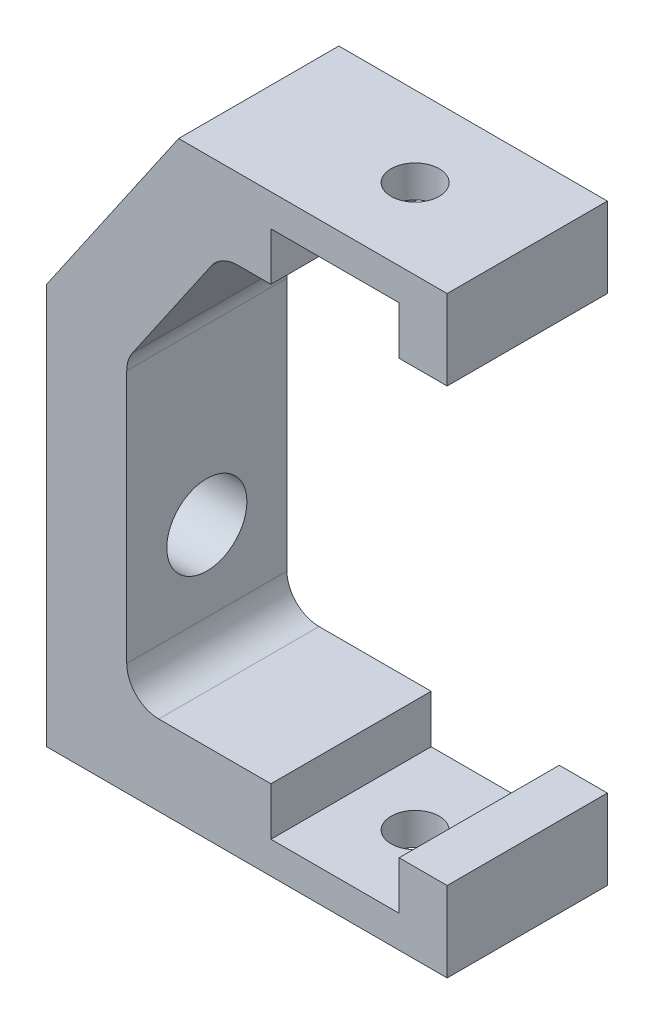
ISO-10303-21;
HEADER;
FILE_DESCRIPTION(('STEP AP214'),'2;1');
FILE_NAME('part.step','',(''),(''),'','','');
FILE_SCHEMA(('AUTOMOTIVE_DESIGN { 1 0 10303 214 1 1 1 1 }'));
ENDSEC;
DATA;
#1=APPLICATION_CONTEXT('core data for automotive mechanical design processes');
#2=APPLICATION_PROTOCOL_DEFINITION('international standard','automotive_design',2000,#1);
#3=PRODUCT_CONTEXT('',#1,'mechanical');
#4=PRODUCT('Part','Part','',(#3));
#5=PRODUCT_RELATED_PRODUCT_CATEGORY('part','',(#4));
#6=PRODUCT_DEFINITION_FORMATION('','',#4);
#7=PRODUCT_DEFINITION_CONTEXT('part definition',#1,'design');
#8=PRODUCT_DEFINITION('design','',#6,#7);
#9=PRODUCT_DEFINITION_SHAPE('','',#8);
#10=(LENGTH_UNIT() NAMED_UNIT(*) SI_UNIT(.MILLI.,.METRE.));
#11=(NAMED_UNIT(*) PLANE_ANGLE_UNIT() SI_UNIT($,.RADIAN.));
#12=(NAMED_UNIT(*) SI_UNIT($,.STERADIAN.) SOLID_ANGLE_UNIT());
#13=UNCERTAINTY_MEASURE_WITH_UNIT(LENGTH_MEASURE(1.E-05),#10,'distance_accuracy_value','');
#14=(GEOMETRIC_REPRESENTATION_CONTEXT(3) GLOBAL_UNCERTAINTY_ASSIGNED_CONTEXT((#13)) GLOBAL_UNIT_ASSIGNED_CONTEXT((#10,
#11,#12)) REPRESENTATION_CONTEXT('',''));
#15=CARTESIAN_POINT('',(0.,0.,0.));
#16=DIRECTION('',(0.,0.,1.));
#17=DIRECTION('',(1.,0.,0.));
#18=AXIS2_PLACEMENT_3D('',#15,#16,#17);
#19=CARTESIAN_POINT('',(25.,0.,5.));
#20=DIRECTION('',(0.,1.,0.));
#21=DIRECTION('',(0.,0.,1.));
#22=AXIS2_PLACEMENT_3D('',#19,#20,#21);
#23=PLANE('',#22);
#24=CARTESIAN_POINT('',(18.,0.,0.));
#25=DIRECTION('',(0.,1.,0.));
#26=DIRECTION('',(0.,0.,1.));
#27=AXIS2_PLACEMENT_3D('',#24,#25,#26);
#28=CIRCLE('',#27,1.5);
#29=CARTESIAN_POINT('',(18.,0.,1.5));
#30=VERTEX_POINT('',#29);
#31=EDGE_CURVE('E388',#30,#30,#28,.T.);
#32=ORIENTED_EDGE('',*,*,#31,.T.);
#33=EDGE_LOOP('',(#32));
#34=FACE_BOUND('',#33,.T.);
#35=DIRECTION('',(1.,0.,0.));
#36=VECTOR('',#35,1.);
#37=CARTESIAN_POINT('',(25.,0.,-5.));
#38=LINE('',#37,#36);
#39=CARTESIAN_POINT('',(0.,0.,-5.));
#40=VERTEX_POINT('',#39);
#41=CARTESIAN_POINT('',(25.,0.,-5.));
#42=VERTEX_POINT('',#41);
#43=EDGE_CURVE('E212',#40,#42,#38,.T.);
#44=ORIENTED_EDGE('',*,*,#43,.T.);
#45=DIRECTION('',(0.,0.,-1.));
#46=VECTOR('',#45,1.);
#47=CARTESIAN_POINT('',(25.,0.,5.));
#48=LINE('',#47,#46);
#49=CARTESIAN_POINT('',(25.,0.,5.));
#50=VERTEX_POINT('',#49);
#51=EDGE_CURVE('E11',#50,#42,#48,.T.);
#52=ORIENTED_EDGE('',*,*,#51,.F.);
#53=DIRECTION('',(1.,0.,0.));
#54=VECTOR('',#53,1.);
#55=CARTESIAN_POINT('',(25.,0.,5.));
#56=LINE('',#55,#54);
#57=CARTESIAN_POINT('',(0.,0.,5.));
#58=VERTEX_POINT('',#57);
#59=EDGE_CURVE('E255',#58,#50,#56,.T.);
#60=ORIENTED_EDGE('',*,*,#59,.F.);
#61=DIRECTION('',(0.,0.,-1.));
#62=VECTOR('',#61,1.);
#63=CARTESIAN_POINT('',(0.,0.,5.));
#64=LINE('',#63,#62);
#65=EDGE_CURVE('E209',#58,#40,#64,.T.);
#66=ORIENTED_EDGE('',*,*,#65,.T.);
#67=EDGE_LOOP('',(#44,#52,#60,#66));
#68=FACE_BOUND('',#67,.T.);
#69=ADVANCED_FACE('F39',(#34,#68),#23,.F.);
#70=CARTESIAN_POINT('',(25.,5.,5.));
#71=DIRECTION('',(-1.,0.,0.));
#72=DIRECTION('',(0.,0.,1.));
#73=AXIS2_PLACEMENT_3D('',#70,#71,#72);
#74=PLANE('',#73);
#75=DIRECTION('',(0.,1.,0.));
#76=VECTOR('',#75,1.);
#77=CARTESIAN_POINT('',(25.,5.,-5.));
#78=LINE('',#77,#76);
#79=CARTESIAN_POINT('',(25.,5.,-5.));
#80=VERTEX_POINT('',#79);
#81=EDGE_CURVE('E220',#42,#80,#78,.T.);
#82=ORIENTED_EDGE('',*,*,#81,.T.);
#83=DIRECTION('',(0.,0.,-1.));
#84=VECTOR('',#83,1.);
#85=CARTESIAN_POINT('',(25.,5.,5.));
#86=LINE('',#85,#84);
#87=CARTESIAN_POINT('',(25.,5.,5.));
#88=VERTEX_POINT('',#87);
#89=EDGE_CURVE('E48',#88,#80,#86,.T.);
#90=ORIENTED_EDGE('',*,*,#89,.F.);
#91=DIRECTION('',(0.,1.,0.));
#92=VECTOR('',#91,1.);
#93=CARTESIAN_POINT('',(25.,5.,5.));
#94=LINE('',#93,#92);
#95=EDGE_CURVE('E137',#50,#88,#94,.T.);
#96=ORIENTED_EDGE('',*,*,#95,.F.);
#97=ORIENTED_EDGE('',*,*,#51,.T.);
#98=EDGE_LOOP('',(#82,#90,#96,#97));
#99=FACE_BOUND('',#98,.T.);
#100=ADVANCED_FACE('F385',(#99),#74,.F.);
#101=CARTESIAN_POINT('',(25.,5.,5.));
#102=DIRECTION('',(0.,-1.,0.));
#103=DIRECTION('',(1.,0.,0.));
#104=AXIS2_PLACEMENT_3D('',#101,#102,#103);
#105=PLANE('',#104);
#106=DIRECTION('',(-1.,0.,0.));
#107=VECTOR('',#106,1.);
#108=CARTESIAN_POINT('',(25.,5.,-5.));
#109=LINE('',#108,#107);
#110=CARTESIAN_POINT('',(22.,5.,-5.));
#111=VERTEX_POINT('',#110);
#112=EDGE_CURVE('E218',#80,#111,#109,.T.);
#113=ORIENTED_EDGE('',*,*,#112,.T.);
#114=DIRECTION('',(0.,0.,-1.));
#115=VECTOR('',#114,1.);
#116=CARTESIAN_POINT('',(22.,5.,5.));
#117=LINE('',#116,#115);
#118=CARTESIAN_POINT('',(22.,5.,5.));
#119=VERTEX_POINT('',#118);
#120=EDGE_CURVE('E300',#119,#111,#117,.T.);
#121=ORIENTED_EDGE('',*,*,#120,.F.);
#122=DIRECTION('',(-1.,0.,0.));
#123=VECTOR('',#122,1.);
#124=CARTESIAN_POINT('',(25.,5.,5.));
#125=LINE('',#124,#123);
#126=EDGE_CURVE('E310',#88,#119,#125,.T.);
#127=ORIENTED_EDGE('',*,*,#126,.F.);
#128=ORIENTED_EDGE('',*,*,#89,.T.);
#129=EDGE_LOOP('',(#113,#121,#127,#128));
#130=FACE_BOUND('',#129,.T.);
#131=ADVANCED_FACE('F307',(#130),#105,.F.);
#132=CARTESIAN_POINT('',(22.,2.,5.));
#133=DIRECTION('',(1.,0.,0.));
#134=DIRECTION('',(0.,0.,-1.));
#135=AXIS2_PLACEMENT_3D('',#132,#133,#134);
#136=PLANE('',#135);
#137=DIRECTION('',(0.,-1.,0.));
#138=VECTOR('',#137,1.);
#139=CARTESIAN_POINT('',(22.,2.,-5.));
#140=LINE('',#139,#138);
#141=CARTESIAN_POINT('',(22.,2.,-5.));
#142=VERTEX_POINT('',#141);
#143=EDGE_CURVE('E222',#111,#142,#140,.T.);
#144=ORIENTED_EDGE('',*,*,#143,.T.);
#145=DIRECTION('',(0.,0.,-1.));
#146=VECTOR('',#145,1.);
#147=CARTESIAN_POINT('',(22.,2.,5.));
#148=LINE('',#147,#146);
#149=CARTESIAN_POINT('',(22.,2.,5.));
#150=VERTEX_POINT('',#149);
#151=EDGE_CURVE('E297',#150,#142,#148,.T.);
#152=ORIENTED_EDGE('',*,*,#151,.F.);
#153=DIRECTION('',(0.,-1.,0.));
#154=VECTOR('',#153,1.);
#155=CARTESIAN_POINT('',(22.,2.,5.));
#156=LINE('',#155,#154);
#157=EDGE_CURVE('E330',#119,#150,#156,.T.);
#158=ORIENTED_EDGE('',*,*,#157,.F.);
#159=ORIENTED_EDGE('',*,*,#120,.T.);
#160=EDGE_LOOP('',(#144,#152,#158,#159));
#161=FACE_BOUND('',#160,.T.);
#162=ADVANCED_FACE('F318',(#161),#136,.F.);
#163=CARTESIAN_POINT('',(14.,2.,5.));
#164=DIRECTION('',(0.,-1.,0.));
#165=DIRECTION('',(0.,0.,-1.));
#166=AXIS2_PLACEMENT_3D('',#163,#164,#165);
#167=PLANE('',#166);
#168=CARTESIAN_POINT('',(18.,2.,0.));
#169=DIRECTION('',(0.,-1.,0.));
#170=DIRECTION('',(0.,0.,-1.));
#171=AXIS2_PLACEMENT_3D('',#168,#169,#170);
#172=CIRCLE('',#171,1.5);
#173=CARTESIAN_POINT('',(18.,2.,-1.5));
#174=VERTEX_POINT('',#173);
#175=EDGE_CURVE('E394',#174,#174,#172,.T.);
#176=ORIENTED_EDGE('',*,*,#175,.T.);
#177=EDGE_LOOP('',(#176));
#178=FACE_BOUND('',#177,.T.);
#179=DIRECTION('',(-1.,0.,0.));
#180=VECTOR('',#179,1.);
#181=CARTESIAN_POINT('',(14.,2.,-5.));
#182=LINE('',#181,#180);
#183=CARTESIAN_POINT('',(14.,2.,-5.));
#184=VERTEX_POINT('',#183);
#185=EDGE_CURVE('E224',#142,#184,#182,.T.);
#186=ORIENTED_EDGE('',*,*,#185,.T.);
#187=DIRECTION('',(0.,0.,-1.));
#188=VECTOR('',#187,1.);
#189=CARTESIAN_POINT('',(14.,2.,5.));
#190=LINE('',#189,#188);
#191=CARTESIAN_POINT('',(14.,2.,5.));
#192=VERTEX_POINT('',#191);
#193=EDGE_CURVE('E294',#192,#184,#190,.T.);
#194=ORIENTED_EDGE('',*,*,#193,.F.);
#195=DIRECTION('',(-1.,0.,0.));
#196=VECTOR('',#195,1.);
#197=CARTESIAN_POINT('',(14.,2.,5.));
#198=LINE('',#197,#196);
#199=EDGE_CURVE('E322',#150,#192,#198,.T.);
#200=ORIENTED_EDGE('',*,*,#199,.F.);
#201=ORIENTED_EDGE('',*,*,#151,.T.);
#202=EDGE_LOOP('',(#186,#194,#200,#201));
#203=FACE_BOUND('',#202,.T.);
#204=ADVANCED_FACE('F325',(#178,#203),#167,.F.);
#205=CARTESIAN_POINT('',(14.,5.,5.));
#206=DIRECTION('',(-1.,0.,0.));
#207=DIRECTION('',(0.,0.,1.));
#208=AXIS2_PLACEMENT_3D('',#205,#206,#207);
#209=PLANE('',#208);
#210=DIRECTION('',(0.,1.,0.));
#211=VECTOR('',#210,1.);
#212=CARTESIAN_POINT('',(14.,5.,-5.));
#213=LINE('',#212,#211);
#214=CARTESIAN_POINT('',(14.,5.,-5.));
#215=VERTEX_POINT('',#214);
#216=EDGE_CURVE('E223',#184,#215,#213,.T.);
#217=ORIENTED_EDGE('',*,*,#216,.T.);
#218=DIRECTION('',(0.,0.,-1.));
#219=VECTOR('',#218,1.);
#220=CARTESIAN_POINT('',(14.,5.,5.));
#221=LINE('',#220,#219);
#222=CARTESIAN_POINT('',(14.,5.,5.));
#223=VERTEX_POINT('',#222);
#224=EDGE_CURVE('E292',#223,#215,#221,.T.);
#225=ORIENTED_EDGE('',*,*,#224,.F.);
#226=DIRECTION('',(0.,1.,0.));
#227=VECTOR('',#226,1.);
#228=CARTESIAN_POINT('',(14.,5.,5.));
#229=LINE('',#228,#227);
#230=EDGE_CURVE('E326',#192,#223,#229,.T.);
#231=ORIENTED_EDGE('',*,*,#230,.F.);
#232=ORIENTED_EDGE('',*,*,#193,.T.);
#233=EDGE_LOOP('',(#217,#225,#231,#232));
#234=FACE_BOUND('',#233,.T.);
#235=ADVANCED_FACE('F458',(#234),#209,.F.);
#236=CARTESIAN_POINT('',(14.,5.,5.));
#237=DIRECTION('',(0.,-1.,0.));
#238=DIRECTION('',(1.,0.,0.));
#239=AXIS2_PLACEMENT_3D('',#236,#237,#238);
#240=PLANE('',#239);
#241=DIRECTION('',(-1.,0.,0.));
#242=VECTOR('',#241,1.);
#243=CARTESIAN_POINT('',(14.,5.,-5.));
#244=LINE('',#243,#242);
#245=CARTESIAN_POINT('',(7.00000000000002,5.,-5.));
#246=VERTEX_POINT('',#245);
#247=EDGE_CURVE('E227',#215,#246,#244,.T.);
#248=ORIENTED_EDGE('',*,*,#247,.T.);
#249=DIRECTION('',(0.,0.,-1.));
#250=VECTOR('',#249,1.);
#251=CARTESIAN_POINT('',(7.00000000000002,5.,5.));
#252=LINE('',#251,#250);
#253=CARTESIAN_POINT('',(7.00000000000002,5.,5.));
#254=VERTEX_POINT('',#253);
#255=EDGE_CURVE('E287',#254,#246,#252,.T.);
#256=ORIENTED_EDGE('',*,*,#255,.F.);
#257=DIRECTION('',(-1.,0.,0.));
#258=VECTOR('',#257,1.);
#259=CARTESIAN_POINT('',(14.,5.,5.));
#260=LINE('',#259,#258);
#261=EDGE_CURVE('E328',#223,#254,#260,.T.);
#262=ORIENTED_EDGE('',*,*,#261,.F.);
#263=ORIENTED_EDGE('',*,*,#224,.T.);
#264=EDGE_LOOP('',(#248,#256,#262,#263));
#265=FACE_BOUND('',#264,.T.);
#266=ADVANCED_FACE('F457',(#265),#240,.F.);
#267=CARTESIAN_POINT('',(7.,7.,5.));
#268=DIRECTION('',(0.,0.,-1.));
#269=DIRECTION('',(-1.,0.,0.));
#270=AXIS2_PLACEMENT_3D('',#267,#268,#269);
#271=CYLINDRICAL_SURFACE('',#270,2.);
#272=CARTESIAN_POINT('',(7.,7.,-5.));
#273=DIRECTION('',(0.,0.,-1.));
#274=DIRECTION('',(-1.,0.,0.));
#275=AXIS2_PLACEMENT_3D('',#272,#273,#274);
#276=CIRCLE('',#275,2.);
#277=CARTESIAN_POINT('',(5.,7.00000000000001,-5.));
#278=VERTEX_POINT('',#277);
#279=EDGE_CURVE('E228',#246,#278,#276,.T.);
#280=ORIENTED_EDGE('',*,*,#279,.T.);
#281=DIRECTION('',(0.,0.,-1.));
#282=VECTOR('',#281,1.);
#283=CARTESIAN_POINT('',(5.,7.00000000000001,5.));
#284=LINE('',#283,#282);
#285=CARTESIAN_POINT('',(5.,7.00000000000001,5.));
#286=VERTEX_POINT('',#285);
#287=EDGE_CURVE('E285',#286,#278,#284,.T.);
#288=ORIENTED_EDGE('',*,*,#287,.F.);
#289=CARTESIAN_POINT('',(7.,7.,5.));
#290=DIRECTION('',(0.,0.,-1.));
#291=DIRECTION('',(-1.,0.,0.));
#292=AXIS2_PLACEMENT_3D('',#289,#290,#291);
#293=CIRCLE('',#292,2.);
#294=EDGE_CURVE('E333',#254,#286,#293,.T.);
#295=ORIENTED_EDGE('',*,*,#294,.F.);
#296=ORIENTED_EDGE('',*,*,#255,.T.);
#297=EDGE_LOOP('',(#280,#288,#295,#296));
#298=FACE_BOUND('',#297,.T.);
#299=ADVANCED_FACE('F454',(#298),#271,.F.);
#300=CARTESIAN_POINT('',(5.,7.00000000000001,5.));
#301=DIRECTION('',(-1.,0.,0.));
#302=DIRECTION('',(0.,0.,1.));
#303=AXIS2_PLACEMENT_3D('',#300,#301,#302);
#304=PLANE('',#303);
#305=CARTESIAN_POINT('',(5.,12.,0.));
#306=DIRECTION('',(1.,0.,0.));
#307=DIRECTION('',(0.,0.,-1.));
#308=AXIS2_PLACEMENT_3D('',#305,#306,#307);
#309=CIRCLE('',#308,2.5);
#310=CARTESIAN_POINT('',(5.,12.,-2.5));
#311=VERTEX_POINT('',#310);
#312=EDGE_CURVE('E392',#311,#311,#309,.T.);
#313=ORIENTED_EDGE('',*,*,#312,.F.);
#314=EDGE_LOOP('',(#313));
#315=FACE_BOUND('',#314,.T.);
#316=DIRECTION('',(0.,1.,0.));
#317=VECTOR('',#316,1.);
#318=CARTESIAN_POINT('',(5.,7.00000000000001,-5.));
#319=LINE('',#318,#317);
#320=CARTESIAN_POINT('',(5.,22.8283399513637,-5.));
#321=VERTEX_POINT('',#320);
#322=EDGE_CURVE('E233',#278,#321,#319,.T.);
#323=ORIENTED_EDGE('',*,*,#322,.T.);
#324=DIRECTION('',(0.,0.,-1.));
#325=VECTOR('',#324,1.);
#326=CARTESIAN_POINT('',(5.,22.8283399513637,5.));
#327=LINE('',#326,#325);
#328=CARTESIAN_POINT('',(5.,22.8283399513637,5.));
#329=VERTEX_POINT('',#328);
#330=EDGE_CURVE('E282',#329,#321,#327,.T.);
#331=ORIENTED_EDGE('',*,*,#330,.F.);
#332=DIRECTION('',(0.,1.,0.));
#333=VECTOR('',#332,1.);
#334=CARTESIAN_POINT('',(5.,7.00000000000001,5.));
#335=LINE('',#334,#333);
#336=EDGE_CURVE('E337',#286,#329,#335,.T.);
#337=ORIENTED_EDGE('',*,*,#336,.F.);
#338=ORIENTED_EDGE('',*,*,#287,.T.);
#339=EDGE_LOOP('',(#323,#331,#337,#338));
#340=FACE_BOUND('',#339,.T.);
#341=ADVANCED_FACE('F448',(#315,#340),#304,.F.);
#342=CARTESIAN_POINT('',(7.,22.8283399513637,5.));
#343=DIRECTION('',(0.,0.,-1.));
#344=DIRECTION('',(-1.,0.,0.));
#345=AXIS2_PLACEMENT_3D('',#342,#343,#344);
#346=CYLINDRICAL_SURFACE('',#345,2.);
#347=CARTESIAN_POINT('',(7.,22.8283399513637,-5.));
#348=DIRECTION('',(0.,0.,-1.));
#349=DIRECTION('',(-1.,0.,0.));
#350=AXIS2_PLACEMENT_3D('',#347,#348,#349);
#351=CIRCLE('',#350,2.);
#352=CARTESIAN_POINT('',(5.35118757467925,23.960337118369,-5.));
#353=VERTEX_POINT('',#352);
#354=EDGE_CURVE('E232',#321,#353,#351,.T.);
#355=ORIENTED_EDGE('',*,*,#354,.T.);
#356=DIRECTION('',(0.,0.,-1.));
#357=VECTOR('',#356,1.);
#358=CARTESIAN_POINT('',(5.35118757467925,23.960337118369,5.));
#359=LINE('',#358,#357);
#360=CARTESIAN_POINT('',(5.35118757467925,23.960337118369,5.));
#361=VERTEX_POINT('',#360);
#362=EDGE_CURVE('E276',#361,#353,#359,.T.);
#363=ORIENTED_EDGE('',*,*,#362,.F.);
#364=CARTESIAN_POINT('',(7.,22.8283399513637,5.));
#365=DIRECTION('',(0.,0.,-1.));
#366=DIRECTION('',(-1.,0.,0.));
#367=AXIS2_PLACEMENT_3D('',#364,#365,#366);
#368=CIRCLE('',#367,2.);
#369=EDGE_CURVE('E338',#329,#361,#368,.T.);
#370=ORIENTED_EDGE('',*,*,#369,.F.);
#371=ORIENTED_EDGE('',*,*,#330,.T.);
#372=EDGE_LOOP('',(#355,#363,#370,#371));
#373=FACE_BOUND('',#372,.T.);
#374=ADVANCED_FACE('F443',(#373),#346,.F.);
#375=CARTESIAN_POINT('',(5.35118757467925,23.960337118369,5.));
#376=DIRECTION('',(-0.824406212660378,0.56599858350262,0.));
#377=DIRECTION('',(-0.56599858350262,-0.824406212660378,0.));
#378=AXIS2_PLACEMENT_3D('',#375,#376,#377);
#379=PLANE('',#378);
#380=DIRECTION('',(0.56599858350262,0.824406212660378,0.));
#381=VECTOR('',#380,1.);
#382=CARTESIAN_POINT('',(5.35118757467925,23.960337118369,-5.));
#383=LINE('',#382,#381);
#384=CARTESIAN_POINT('',(10.2749125133736,31.1319971670052,-5.));
#385=VERTEX_POINT('',#384);
#386=EDGE_CURVE('E231',#353,#385,#383,.T.);
#387=ORIENTED_EDGE('',*,*,#386,.T.);
#388=DIRECTION('',(0.,0.,-1.));
#389=VECTOR('',#388,1.);
#390=CARTESIAN_POINT('',(10.2749125133736,31.1319971670052,5.));
#391=LINE('',#390,#389);
#392=CARTESIAN_POINT('',(10.2749125133736,31.1319971670052,5.));
#393=VERTEX_POINT('',#392);
#394=EDGE_CURVE('E277',#393,#385,#391,.T.);
#395=ORIENTED_EDGE('',*,*,#394,.F.);
#396=DIRECTION('',(0.56599858350262,0.824406212660378,0.));
#397=VECTOR('',#396,1.);
#398=CARTESIAN_POINT('',(5.35118757467925,23.960337118369,5.));
#399=LINE('',#398,#397);
#400=EDGE_CURVE('E343',#361,#393,#399,.T.);
#401=ORIENTED_EDGE('',*,*,#400,.F.);
#402=ORIENTED_EDGE('',*,*,#362,.T.);
#403=EDGE_LOOP('',(#387,#395,#401,#402));
#404=FACE_BOUND('',#403,.T.);
#405=ADVANCED_FACE('F442',(#404),#379,.F.);
#406=CARTESIAN_POINT('',(11.9237249386943,30.,5.));
#407=DIRECTION('',(0.,0.,-1.));
#408=DIRECTION('',(-1.,0.,0.));
#409=AXIS2_PLACEMENT_3D('',#406,#407,#408);
#410=CYLINDRICAL_SURFACE('',#409,2.);
#411=CARTESIAN_POINT('',(11.9237249386943,30.,-5.));
#412=DIRECTION('',(0.,0.,-1.));
#413=DIRECTION('',(1.,0.,0.));
#414=AXIS2_PLACEMENT_3D('',#411,#412,#413);
#415=CIRCLE('',#414,2.);
#416=CARTESIAN_POINT('',(11.9237249386944,32.,-5.));
#417=VERTEX_POINT('',#416);
#418=EDGE_CURVE('E240',#385,#417,#415,.T.);
#419=ORIENTED_EDGE('',*,*,#418,.T.);
#420=DIRECTION('',(0.,0.,-1.));
#421=VECTOR('',#420,1.);
#422=CARTESIAN_POINT('',(11.9237249386944,32.,5.));
#423=LINE('',#422,#421);
#424=CARTESIAN_POINT('',(11.9237249386944,32.,5.));
#425=VERTEX_POINT('',#424);
#426=EDGE_CURVE('E272',#425,#417,#423,.T.);
#427=ORIENTED_EDGE('',*,*,#426,.F.);
#428=CARTESIAN_POINT('',(11.9237249386943,30.,5.));
#429=DIRECTION('',(0.,0.,-1.));
#430=DIRECTION('',(1.,0.,0.));
#431=AXIS2_PLACEMENT_3D('',#428,#429,#430);
#432=CIRCLE('',#431,2.);
#433=EDGE_CURVE('E342',#393,#425,#432,.T.);
#434=ORIENTED_EDGE('',*,*,#433,.F.);
#435=ORIENTED_EDGE('',*,*,#394,.T.);
#436=EDGE_LOOP('',(#419,#427,#434,#435));
#437=FACE_BOUND('',#436,.T.);
#438=ADVANCED_FACE('F440',(#437),#410,.F.);
#439=CARTESIAN_POINT('',(11.9237249386944,32.,5.));
#440=DIRECTION('',(0.,1.,0.));
#441=DIRECTION('',(0.,0.,1.));
#442=AXIS2_PLACEMENT_3D('',#439,#440,#441);
#443=PLANE('',#442);
#444=DIRECTION('',(1.,0.,0.));
#445=VECTOR('',#444,1.);
#446=CARTESIAN_POINT('',(11.9237249386944,32.,-5.));
#447=LINE('',#446,#445);
#448=CARTESIAN_POINT('',(14.,32.,-5.));
#449=VERTEX_POINT('',#448);
#450=EDGE_CURVE('E239',#417,#449,#447,.T.);
#451=ORIENTED_EDGE('',*,*,#450,.T.);
#452=DIRECTION('',(0.,0.,-1.));
#453=VECTOR('',#452,1.);
#454=CARTESIAN_POINT('',(14.,32.,5.));
#455=LINE('',#454,#453);
#456=CARTESIAN_POINT('',(14.,32.,5.));
#457=VERTEX_POINT('',#456);
#458=EDGE_CURVE('E269',#457,#449,#455,.T.);
#459=ORIENTED_EDGE('',*,*,#458,.F.);
#460=DIRECTION('',(1.,0.,0.));
#461=VECTOR('',#460,1.);
#462=CARTESIAN_POINT('',(11.9237249386944,32.,5.));
#463=LINE('',#462,#461);
#464=EDGE_CURVE('E341',#425,#457,#463,.T.);
#465=ORIENTED_EDGE('',*,*,#464,.F.);
#466=ORIENTED_EDGE('',*,*,#426,.T.);
#467=EDGE_LOOP('',(#451,#459,#465,#466));
#468=FACE_BOUND('',#467,.T.);
#469=ADVANCED_FACE('F433',(#468),#443,.F.);
#470=CARTESIAN_POINT('',(14.,35.,5.));
#471=DIRECTION('',(-1.,0.,0.));
#472=DIRECTION('',(0.,0.,1.));
#473=AXIS2_PLACEMENT_3D('',#470,#471,#472);
#474=PLANE('',#473);
#475=DIRECTION('',(0.,1.,0.));
#476=VECTOR('',#475,1.);
#477=CARTESIAN_POINT('',(14.,35.,-5.));
#478=LINE('',#477,#476);
#479=CARTESIAN_POINT('',(14.,35.,-5.));
#480=VERTEX_POINT('',#479);
#481=EDGE_CURVE('E241',#449,#480,#478,.T.);
#482=ORIENTED_EDGE('',*,*,#481,.T.);
#483=DIRECTION('',(0.,0.,-1.));
#484=VECTOR('',#483,1.);
#485=CARTESIAN_POINT('',(14.,35.,5.));
#486=LINE('',#485,#484);
#487=CARTESIAN_POINT('',(14.,35.,5.));
#488=VERTEX_POINT('',#487);
#489=EDGE_CURVE('E270',#488,#480,#486,.T.);
#490=ORIENTED_EDGE('',*,*,#489,.F.);
#491=DIRECTION('',(0.,1.,0.));
#492=VECTOR('',#491,1.);
#493=CARTESIAN_POINT('',(14.,35.,5.));
#494=LINE('',#493,#492);
#495=EDGE_CURVE('E350',#457,#488,#494,.T.);
#496=ORIENTED_EDGE('',*,*,#495,.F.);
#497=ORIENTED_EDGE('',*,*,#458,.T.);
#498=EDGE_LOOP('',(#482,#490,#496,#497));
#499=FACE_BOUND('',#498,.T.);
#500=ADVANCED_FACE('F427',(#499),#474,.F.);
#501=CARTESIAN_POINT('',(22.,35.,5.));
#502=DIRECTION('',(0.,1.,0.));
#503=DIRECTION('',(0.,0.,1.));
#504=AXIS2_PLACEMENT_3D('',#501,#502,#503);
#505=PLANE('',#504);
#506=CARTESIAN_POINT('',(18.,35.,0.));
#507=DIRECTION('',(0.,1.,0.));
#508=DIRECTION('',(0.,0.,1.));
#509=AXIS2_PLACEMENT_3D('',#506,#507,#508);
#510=CIRCLE('',#509,1.5);
#511=CARTESIAN_POINT('',(18.,35.,1.5));
#512=VERTEX_POINT('',#511);
#513=EDGE_CURVE('E397',#512,#512,#510,.T.);
#514=ORIENTED_EDGE('',*,*,#513,.T.);
#515=EDGE_LOOP('',(#514));
#516=FACE_BOUND('',#515,.T.);
#517=DIRECTION('',(1.,0.,0.));
#518=VECTOR('',#517,1.);
#519=CARTESIAN_POINT('',(22.,35.,-5.));
#520=LINE('',#519,#518);
#521=CARTESIAN_POINT('',(22.,35.,-5.));
#522=VERTEX_POINT('',#521);
#523=EDGE_CURVE('E244',#480,#522,#520,.T.);
#524=ORIENTED_EDGE('',*,*,#523,.T.);
#525=DIRECTION('',(0.,0.,-1.));
#526=VECTOR('',#525,1.);
#527=CARTESIAN_POINT('',(22.,35.,5.));
#528=LINE('',#527,#526);
#529=CARTESIAN_POINT('',(22.,35.,5.));
#530=VERTEX_POINT('',#529);
#531=EDGE_CURVE('E262',#530,#522,#528,.T.);
#532=ORIENTED_EDGE('',*,*,#531,.F.);
#533=DIRECTION('',(1.,0.,0.));
#534=VECTOR('',#533,1.);
#535=CARTESIAN_POINT('',(22.,35.,5.));
#536=LINE('',#535,#534);
#537=EDGE_CURVE('E349',#488,#530,#536,.T.);
#538=ORIENTED_EDGE('',*,*,#537,.F.);
#539=ORIENTED_EDGE('',*,*,#489,.T.);
#540=EDGE_LOOP('',(#524,#532,#538,#539));
#541=FACE_BOUND('',#540,.T.);
#542=ADVANCED_FACE('F426',(#516,#541),#505,.F.);
#543=CARTESIAN_POINT('',(22.,32.,5.));
#544=DIRECTION('',(1.,0.,0.));
#545=DIRECTION('',(0.,0.,-1.));
#546=AXIS2_PLACEMENT_3D('',#543,#544,#545);
#547=PLANE('',#546);
#548=DIRECTION('',(0.,-1.,0.));
#549=VECTOR('',#548,1.);
#550=CARTESIAN_POINT('',(22.,32.,-5.));
#551=LINE('',#550,#549);
#552=CARTESIAN_POINT('',(22.,32.,-5.));
#553=VERTEX_POINT('',#552);
#554=EDGE_CURVE('E245',#522,#553,#551,.T.);
#555=ORIENTED_EDGE('',*,*,#554,.T.);
#556=DIRECTION('',(0.,0.,-1.));
#557=VECTOR('',#556,1.);
#558=CARTESIAN_POINT('',(22.,32.,5.));
#559=LINE('',#558,#557);
#560=CARTESIAN_POINT('',(22.,32.,5.));
#561=VERTEX_POINT('',#560);
#562=EDGE_CURVE('E261',#561,#553,#559,.T.);
#563=ORIENTED_EDGE('',*,*,#562,.F.);
#564=DIRECTION('',(0.,-1.,0.));
#565=VECTOR('',#564,1.);
#566=CARTESIAN_POINT('',(22.,32.,5.));
#567=LINE('',#566,#565);
#568=EDGE_CURVE('E351',#530,#561,#567,.T.);
#569=ORIENTED_EDGE('',*,*,#568,.F.);
#570=ORIENTED_EDGE('',*,*,#531,.T.);
#571=EDGE_LOOP('',(#555,#563,#569,#570));
#572=FACE_BOUND('',#571,.T.);
#573=ADVANCED_FACE('F421',(#572),#547,.F.);
#574=CARTESIAN_POINT('',(22.,32.,5.));
#575=DIRECTION('',(0.,1.,0.));
#576=DIRECTION('',(0.,0.,1.));
#577=AXIS2_PLACEMENT_3D('',#574,#575,#576);
#578=PLANE('',#577);
#579=DIRECTION('',(1.,0.,0.));
#580=VECTOR('',#579,1.);
#581=CARTESIAN_POINT('',(22.,32.,-5.));
#582=LINE('',#581,#580);
#583=CARTESIAN_POINT('',(25.,32.,-5.));
#584=VERTEX_POINT('',#583);
#585=EDGE_CURVE('E249',#553,#584,#582,.T.);
#586=ORIENTED_EDGE('',*,*,#585,.T.);
#587=DIRECTION('',(0.,0.,-1.));
#588=VECTOR('',#587,1.);
#589=CARTESIAN_POINT('',(25.,32.,5.));
#590=LINE('',#589,#588);
#591=CARTESIAN_POINT('',(25.,32.,5.));
#592=VERTEX_POINT('',#591);
#593=EDGE_CURVE('E256',#592,#584,#590,.T.);
#594=ORIENTED_EDGE('',*,*,#593,.F.);
#595=DIRECTION('',(1.,0.,0.));
#596=VECTOR('',#595,1.);
#597=CARTESIAN_POINT('',(22.,32.,5.));
#598=LINE('',#597,#596);
#599=EDGE_CURVE('E354',#561,#592,#598,.T.);
#600=ORIENTED_EDGE('',*,*,#599,.F.);
#601=ORIENTED_EDGE('',*,*,#562,.T.);
#602=EDGE_LOOP('',(#586,#594,#600,#601));
#603=FACE_BOUND('',#602,.T.);
#604=ADVANCED_FACE('F360',(#603),#578,.F.);
#605=CARTESIAN_POINT('',(25.,37.,5.));
#606=DIRECTION('',(-1.,0.,0.));
#607=DIRECTION('',(0.,0.,1.));
#608=AXIS2_PLACEMENT_3D('',#605,#606,#607);
#609=PLANE('',#608);
#610=DIRECTION('',(0.,1.,0.));
#611=VECTOR('',#610,1.);
#612=CARTESIAN_POINT('',(25.,37.,-5.));
#613=LINE('',#612,#611);
#614=CARTESIAN_POINT('',(25.,37.,-5.));
#615=VERTEX_POINT('',#614);
#616=EDGE_CURVE('E250',#584,#615,#613,.T.);
#617=ORIENTED_EDGE('',*,*,#616,.T.);
#618=DIRECTION('',(0.,0.,-1.));
#619=VECTOR('',#618,1.);
#620=CARTESIAN_POINT('',(25.,37.,5.));
#621=LINE('',#620,#619);
#622=CARTESIAN_POINT('',(25.,37.,5.));
#623=VERTEX_POINT('',#622);
#624=EDGE_CURVE('E202',#623,#615,#621,.T.);
#625=ORIENTED_EDGE('',*,*,#624,.F.);
#626=DIRECTION('',(0.,1.,0.));
#627=VECTOR('',#626,1.);
#628=CARTESIAN_POINT('',(25.,37.,5.));
#629=LINE('',#628,#627);
#630=EDGE_CURVE('E198',#592,#623,#629,.T.);
#631=ORIENTED_EDGE('',*,*,#630,.F.);
#632=ORIENTED_EDGE('',*,*,#593,.T.);
#633=EDGE_LOOP('',(#617,#625,#631,#632));
#634=FACE_BOUND('',#633,.T.);
#635=ADVANCED_FACE('F361',(#634),#609,.F.);
#636=CARTESIAN_POINT('',(8.23863636363626,37.,5.));
#637=DIRECTION('',(0.,-1.,0.));
#638=DIRECTION('',(0.,0.,-1.));
#639=AXIS2_PLACEMENT_3D('',#636,#637,#638);
#640=PLANE('',#639);
#641=CARTESIAN_POINT('',(18.,37.,0.));
#642=DIRECTION('',(0.,1.,0.));
#643=DIRECTION('',(0.,0.,1.));
#644=AXIS2_PLACEMENT_3D('',#641,#642,#643);
#645=CIRCLE('',#644,1.5);
#646=CARTESIAN_POINT('',(18.,37.,1.5));
#647=VERTEX_POINT('',#646);
#648=EDGE_CURVE('E403',#647,#647,#645,.T.);
#649=ORIENTED_EDGE('',*,*,#648,.F.);
#650=EDGE_LOOP('',(#649));
#651=FACE_BOUND('',#650,.T.);
#652=DIRECTION('',(-1.,0.,0.));
#653=VECTOR('',#652,1.);
#654=CARTESIAN_POINT('',(8.23863636363626,37.,-5.));
#655=LINE('',#654,#653);
#656=CARTESIAN_POINT('',(8.23863636363626,37.,-5.));
#657=VERTEX_POINT('',#656);
#658=EDGE_CURVE('E204',#615,#657,#655,.T.);
#659=ORIENTED_EDGE('',*,*,#658,.T.);
#660=DIRECTION('',(0.,0.,-1.));
#661=VECTOR('',#660,1.);
#662=CARTESIAN_POINT('',(8.23863636363626,37.,5.));
#663=LINE('',#662,#661);
#664=CARTESIAN_POINT('',(8.23863636363626,37.,5.));
#665=VERTEX_POINT('',#664);
#666=EDGE_CURVE('E203',#665,#657,#663,.T.);
#667=ORIENTED_EDGE('',*,*,#666,.F.);
#668=DIRECTION('',(-1.,0.,0.));
#669=VECTOR('',#668,1.);
#670=CARTESIAN_POINT('',(8.23863636363626,37.,5.));
#671=LINE('',#670,#669);
#672=EDGE_CURVE('E190',#623,#665,#671,.T.);
#673=ORIENTED_EDGE('',*,*,#672,.F.);
#674=ORIENTED_EDGE('',*,*,#624,.T.);
#675=EDGE_LOOP('',(#659,#667,#673,#674));
#676=FACE_BOUND('',#675,.T.);
#677=ADVANCED_FACE('F205',(#651,#676),#640,.F.);
#678=CARTESIAN_POINT('',(0.,25.,5.));
#679=DIRECTION('',(0.824406212660378,-0.56599858350262,0.));
#680=DIRECTION('',(0.56599858350262,0.824406212660378,0.));
#681=AXIS2_PLACEMENT_3D('',#678,#679,#680);
#682=PLANE('',#681);
#683=DIRECTION('',(-0.56599858350262,-0.824406212660378,0.));
#684=VECTOR('',#683,1.);
#685=CARTESIAN_POINT('',(0.,25.,-5.));
#686=LINE('',#685,#684);
#687=CARTESIAN_POINT('',(0.,25.,-5.));
#688=VERTEX_POINT('',#687);
#689=EDGE_CURVE('E125',#657,#688,#686,.T.);
#690=ORIENTED_EDGE('',*,*,#689,.T.);
#691=DIRECTION('',(0.,0.,-1.));
#692=VECTOR('',#691,1.);
#693=CARTESIAN_POINT('',(0.,25.,5.));
#694=LINE('',#693,#692);
#695=CARTESIAN_POINT('',(0.,25.,5.));
#696=VERTEX_POINT('',#695);
#697=EDGE_CURVE('E206',#696,#688,#694,.T.);
#698=ORIENTED_EDGE('',*,*,#697,.F.);
#699=DIRECTION('',(-0.56599858350262,-0.824406212660378,0.));
#700=VECTOR('',#699,1.);
#701=CARTESIAN_POINT('',(0.,25.,5.));
#702=LINE('',#701,#700);
#703=EDGE_CURVE('E195',#665,#696,#702,.T.);
#704=ORIENTED_EDGE('',*,*,#703,.F.);
#705=ORIENTED_EDGE('',*,*,#666,.T.);
#706=EDGE_LOOP('',(#690,#698,#704,#705));
#707=FACE_BOUND('',#706,.T.);
#708=ADVANCED_FACE('F208',(#707),#682,.F.);
#709=CARTESIAN_POINT('',(0.,0.,5.));
#710=DIRECTION('',(1.,0.,0.));
#711=DIRECTION('',(0.,1.,0.));
#712=AXIS2_PLACEMENT_3D('',#709,#710,#711);
#713=PLANE('',#712);
#714=CARTESIAN_POINT('',(0.,12.,0.));
#715=DIRECTION('',(1.,0.,0.));
#716=DIRECTION('',(0.,1.,0.));
#717=AXIS2_PLACEMENT_3D('',#714,#715,#716);
#718=CIRCLE('',#717,2.5);
#719=CARTESIAN_POINT('',(0.,14.5,0.));
#720=VERTEX_POINT('',#719);
#721=EDGE_CURVE('E45',#720,#720,#718,.T.);
#722=ORIENTED_EDGE('',*,*,#721,.T.);
#723=EDGE_LOOP('',(#722));
#724=FACE_BOUND('',#723,.T.);
#725=DIRECTION('',(0.,-1.,0.));
#726=VECTOR('',#725,1.);
#727=CARTESIAN_POINT('',(0.,0.,-5.));
#728=LINE('',#727,#726);
#729=EDGE_CURVE('E128',#688,#40,#728,.T.);
#730=ORIENTED_EDGE('',*,*,#729,.T.);
#731=ORIENTED_EDGE('',*,*,#65,.F.);
#732=DIRECTION('',(0.,-1.,0.));
#733=VECTOR('',#732,1.);
#734=CARTESIAN_POINT('',(0.,0.,5.));
#735=LINE('',#734,#733);
#736=EDGE_CURVE('E57',#696,#58,#735,.T.);
#737=ORIENTED_EDGE('',*,*,#736,.F.);
#738=ORIENTED_EDGE('',*,*,#697,.T.);
#739=EDGE_LOOP('',(#730,#731,#737,#738));
#740=FACE_BOUND('',#739,.T.);
#741=ADVANCED_FACE('F370',(#724,#740),#713,.F.);
#742=CARTESIAN_POINT('',(11.9237249386943,30.,5.));
#743=DIRECTION('',(0.,0.,1.));
#744=DIRECTION('',(1.,0.,0.));
#745=AXIS2_PLACEMENT_3D('',#742,#743,#744);
#746=PLANE('',#745);
#747=ORIENTED_EDGE('',*,*,#59,.T.);
#748=ORIENTED_EDGE('',*,*,#95,.T.);
#749=ORIENTED_EDGE('',*,*,#126,.T.);
#750=ORIENTED_EDGE('',*,*,#157,.T.);
#751=ORIENTED_EDGE('',*,*,#199,.T.);
#752=ORIENTED_EDGE('',*,*,#230,.T.);
#753=ORIENTED_EDGE('',*,*,#261,.T.);
#754=ORIENTED_EDGE('',*,*,#294,.T.);
#755=ORIENTED_EDGE('',*,*,#336,.T.);
#756=ORIENTED_EDGE('',*,*,#369,.T.);
#757=ORIENTED_EDGE('',*,*,#400,.T.);
#758=ORIENTED_EDGE('',*,*,#433,.T.);
#759=ORIENTED_EDGE('',*,*,#464,.T.);
#760=ORIENTED_EDGE('',*,*,#495,.T.);
#761=ORIENTED_EDGE('',*,*,#537,.T.);
#762=ORIENTED_EDGE('',*,*,#568,.T.);
#763=ORIENTED_EDGE('',*,*,#599,.T.);
#764=ORIENTED_EDGE('',*,*,#630,.T.);
#765=ORIENTED_EDGE('',*,*,#672,.T.);
#766=ORIENTED_EDGE('',*,*,#703,.T.);
#767=ORIENTED_EDGE('',*,*,#736,.T.);
#768=EDGE_LOOP('',(#747,#748,#749,#750,#751,#752,#753,#754,#755,#756,#757,#758,#759,#760,#761,
#762,#763,#764,#765,#766,#767));
#769=FACE_BOUND('',#768,.T.);
#770=ADVANCED_FACE('F194',(#769),#746,.T.);
#771=CARTESIAN_POINT('',(11.9237249386943,30.,-5.));
#772=DIRECTION('',(0.,0.,1.));
#773=DIRECTION('',(1.,0.,0.));
#774=AXIS2_PLACEMENT_3D('',#771,#772,#773);
#775=PLANE('',#774);
#776=ORIENTED_EDGE('',*,*,#43,.F.);
#777=ORIENTED_EDGE('',*,*,#729,.F.);
#778=ORIENTED_EDGE('',*,*,#689,.F.);
#779=ORIENTED_EDGE('',*,*,#658,.F.);
#780=ORIENTED_EDGE('',*,*,#616,.F.);
#781=ORIENTED_EDGE('',*,*,#585,.F.);
#782=ORIENTED_EDGE('',*,*,#554,.F.);
#783=ORIENTED_EDGE('',*,*,#523,.F.);
#784=ORIENTED_EDGE('',*,*,#481,.F.);
#785=ORIENTED_EDGE('',*,*,#450,.F.);
#786=ORIENTED_EDGE('',*,*,#418,.F.);
#787=ORIENTED_EDGE('',*,*,#386,.F.);
#788=ORIENTED_EDGE('',*,*,#354,.F.);
#789=ORIENTED_EDGE('',*,*,#322,.F.);
#790=ORIENTED_EDGE('',*,*,#279,.F.);
#791=ORIENTED_EDGE('',*,*,#247,.F.);
#792=ORIENTED_EDGE('',*,*,#216,.F.);
#793=ORIENTED_EDGE('',*,*,#185,.F.);
#794=ORIENTED_EDGE('',*,*,#143,.F.);
#795=ORIENTED_EDGE('',*,*,#112,.F.);
#796=ORIENTED_EDGE('',*,*,#81,.F.);
#797=EDGE_LOOP('',(#776,#777,#778,#779,#780,#781,#782,#783,#784,#785,#786,#787,#788,#789,#790,
#791,#792,#793,#794,#795,#796));
#798=FACE_BOUND('',#797,.T.);
#799=ADVANCED_FACE('F311',(#798),#775,.F.);
#800=CARTESIAN_POINT('',(-5.,12.,0.));
#801=DIRECTION('',(1.,0.,0.));
#802=DIRECTION('',(0.,0.,-1.));
#803=AXIS2_PLACEMENT_3D('',#800,#801,#802);
#804=CYLINDRICAL_SURFACE('',#803,2.5);
#805=ORIENTED_EDGE('',*,*,#312,.T.);
#806=EDGE_LOOP('',(#805));
#807=FACE_BOUND('',#806,.T.);
#808=ORIENTED_EDGE('',*,*,#721,.F.);
#809=EDGE_LOOP('',(#808));
#810=FACE_BOUND('',#809,.T.);
#811=ADVANCED_FACE('F554',(#807,#810),#804,.F.);
#812=CARTESIAN_POINT('',(18.,-14.,0.));
#813=DIRECTION('',(0.,1.,0.));
#814=DIRECTION('',(0.,0.,1.));
#815=AXIS2_PLACEMENT_3D('',#812,#813,#814);
#816=CYLINDRICAL_SURFACE('',#815,1.5);
#817=ORIENTED_EDGE('',*,*,#648,.T.);
#818=EDGE_LOOP('',(#817));
#819=FACE_BOUND('',#818,.T.);
#820=ORIENTED_EDGE('',*,*,#513,.F.);
#821=EDGE_LOOP('',(#820));
#822=FACE_BOUND('',#821,.T.);
#823=ADVANCED_FACE('F408',(#819,#822),#816,.F.);
#824=ORIENTED_EDGE('',*,*,#175,.F.);
#825=EDGE_LOOP('',(#824));
#826=FACE_BOUND('',#825,.T.);
#827=ORIENTED_EDGE('',*,*,#31,.F.);
#828=EDGE_LOOP('',(#827));
#829=FACE_BOUND('',#828,.T.);
#830=ADVANCED_FACE('F600',(#826,#829),#816,.F.);
#831=CLOSED_SHELL('',(#69,#100,#131,#162,#204,#235,#266,#299,#341,#374,#405,#438,#469,#500,#542,
#573,#604,#635,#677,#708,#741,#770,#799,#811,#823,#830));
#832=MANIFOLD_SOLID_BREP('B2',#831);
#833=ADVANCED_BREP_SHAPE_REPRESENTATION('',(#18,#832),#14);
#834=SHAPE_DEFINITION_REPRESENTATION(#9,#833);
ENDSEC;
END-ISO-10303-21;
